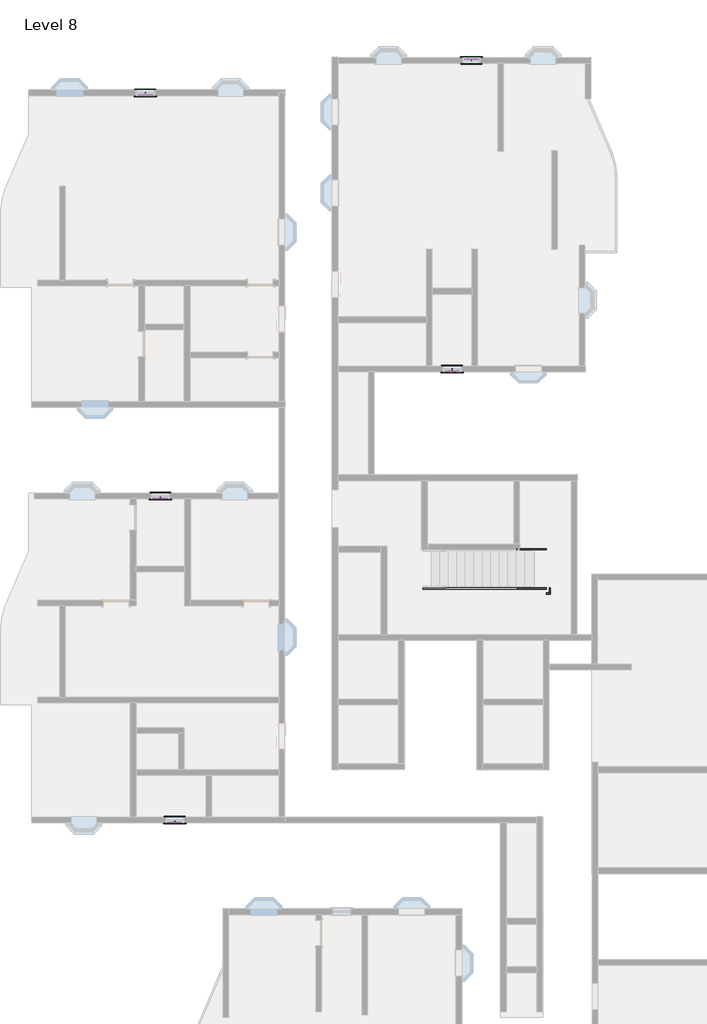
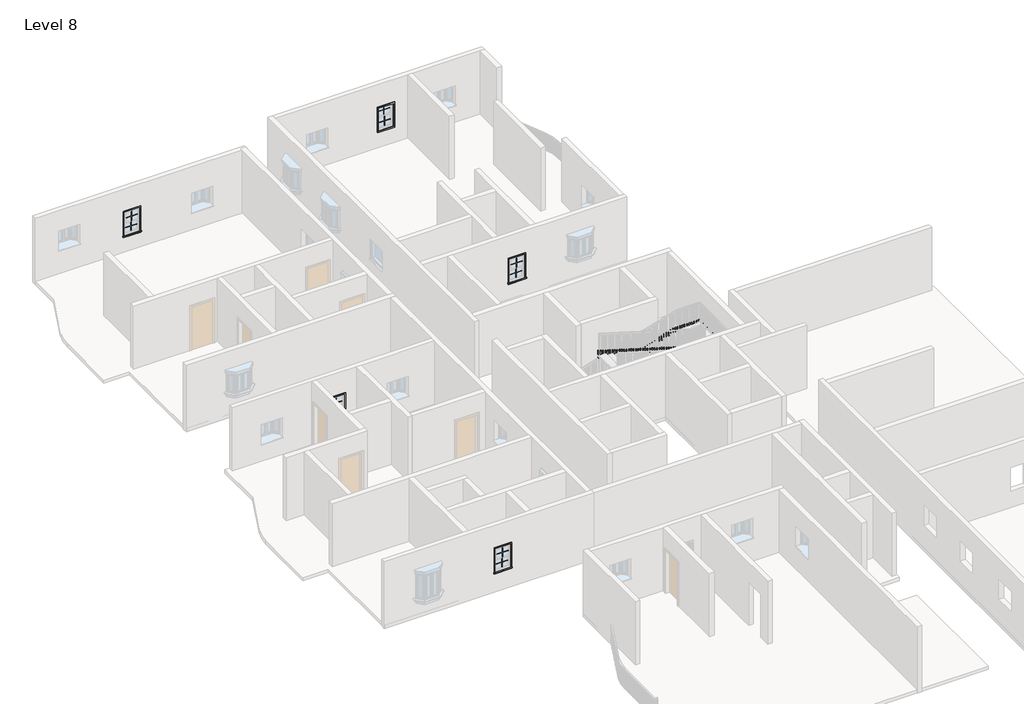
# One storey, part 14 of 14: 20 proxies, 6 members.
"""IFC4 building model written with IfcOpenShell, lengths in millimetres."""

from ifc_helpers import new_model, si_unit, frame, origin, place, context, project, spatial, polyline, outline, extrude, transform, mapped, element, save
from components import muntin_pattern_2x2_muntin_pattern_2x2_c35c595f, trim_window_exterior_flat_with_sill_e38017c9, trim_window_interior_flat_picture_frame_d728ed12

model = new_model("IFC4")

# Units and contexts
model_context = context("Model", 3, world=origin())
ifc_project = project(units=[si_unit("LENGTHUNIT", "METRE", prefix="MILLI")], contexts=[model_context])

# Site, building, storey
site = spatial("IfcSite", under=ifc_project)
building = spatial("IfcBuilding", under=site)
storey = spatial("IfcBuildingStorey", under=building, Name="Level 8", Elevation=21336.0)

# Proxies
placement = place(None, origin())
muntin_pattern_2x2_muntin_pattern_2x2_shape = muntin_pattern_2x2_muntin_pattern_2x2_c35c595f(model_context)
element("IfcBuildingElementProxy", 1, Name="Muntin Pattern_2x2 : Muntin Pattern_2x2", ObjectType="Muntin Pattern_2x2 : Muntin Pattern_2x2", at=placement, inside=storey, context=model_context, shape_type="MappedRepresentation", body=[
    mapped(muntin_pattern_2x2_muntin_pattern_2x2_shape, transform((-14639.3891351, 14368.0833494, 22806.025), x_axis=(-1.0, 0.0, 0.0), y_axis=(0.0, -1.0, 0.0), z_axis=(0.0, 0.0, 1.0))),
])
element("IfcBuildingElementProxy", 2, Name="Muntin Pattern_2x2 : Muntin Pattern_2x2", ObjectType="Muntin Pattern_2x2 : Muntin Pattern_2x2", at=placement, inside=storey, context=model_context, shape_type="MappedRepresentation", body=[
    mapped(muntin_pattern_2x2_muntin_pattern_2x2_shape, transform((-14639.3891351, 14412.5333494, 22326.6), x_axis=(-1.0, 0.0, 0.0), y_axis=(0.0, -1.0, 0.0), z_axis=(0.0, 0.0, 1.0))),
])
element("IfcBuildingElementProxy", 3, Name="Muntin Pattern_2x2 : Muntin Pattern_2x2", ObjectType="Muntin Pattern_2x2 : Muntin Pattern_2x2", at=placement, inside=storey, context=model_context, shape_type="MappedRepresentation", body=[
    mapped(muntin_pattern_2x2_muntin_pattern_2x2_shape, transform((-14125.0391351, 2785.6833494, 22806.025), x_axis=(-1.0, 0.0, 0.0), y_axis=(0.0, -1.0, 0.0), z_axis=(0.0, 0.0, 1.0))),
])
element("IfcBuildingElementProxy", 4, Name="Muntin Pattern_2x2 : Muntin Pattern_2x2", ObjectType="Muntin Pattern_2x2 : Muntin Pattern_2x2", at=placement, inside=storey, context=model_context, shape_type="MappedRepresentation", body=[
    mapped(muntin_pattern_2x2_muntin_pattern_2x2_shape, transform((-14125.0391351, 2830.1333494, 22326.6), x_axis=(-1.0, 0.0, 0.0), y_axis=(0.0, -1.0, 0.0), z_axis=(0.0, 0.0, 1.0))),
])
element("IfcBuildingElementProxy", 5, Name="Muntin Pattern_2x2 : Muntin Pattern_2x2", ObjectType="Muntin Pattern_2x2 : Muntin Pattern_2x2", at=placement, inside=storey, context=model_context, shape_type="MappedRepresentation", body=[
    mapped(muntin_pattern_2x2_muntin_pattern_2x2_shape, transform((-4206.3391351, 18910.0465905, 22806.025), x_axis=(-1.0, 0.0, 0.0), y_axis=(0.0, -1.0, 0.0), z_axis=(0.0, 0.0, 1.0))),
])
element("IfcBuildingElementProxy", 6, Name="Muntin Pattern_2x2 : Muntin Pattern_2x2", ObjectType="Muntin Pattern_2x2 : Muntin Pattern_2x2", at=placement, inside=storey, context=model_context, shape_type="MappedRepresentation", body=[
    mapped(muntin_pattern_2x2_muntin_pattern_2x2_shape, transform((-4206.3391351, 18954.4965905, 22326.6), x_axis=(-1.0, 0.0, 0.0), y_axis=(0.0, -1.0, 0.0), z_axis=(0.0, 0.0, 1.0))),
])
element("IfcBuildingElementProxy", 7, Name="Muntin Pattern_2x2 : Muntin Pattern_2x2", ObjectType="Muntin Pattern_2x2 : Muntin Pattern_2x2", at=placement, inside=storey, context=model_context, shape_type="MappedRepresentation", body=[
    mapped(muntin_pattern_2x2_muntin_pattern_2x2_shape, transform((-3514.1891351, 30066.9965905, 22806.025), x_axis=(1.0, 0.0, 0.0), y_axis=(0.0, 1.0, 0.0), z_axis=(0.0, 0.0, 1.0))),
])
element("IfcBuildingElementProxy", 8, Name="Muntin Pattern_2x2 : Muntin Pattern_2x2", ObjectType="Muntin Pattern_2x2 : Muntin Pattern_2x2", at=placement, inside=storey, context=model_context, shape_type="MappedRepresentation", body=[
    mapped(muntin_pattern_2x2_muntin_pattern_2x2_shape, transform((-3514.1891351, 30022.5465905, 22326.6), x_axis=(1.0, 0.0, 0.0), y_axis=(0.0, 1.0, 0.0), z_axis=(0.0, 0.0, 1.0))),
])
element("IfcBuildingElementProxy", 9, Name="Muntin Pattern_2x2 : Muntin Pattern_2x2", ObjectType="Muntin Pattern_2x2 : Muntin Pattern_2x2", at=placement, inside=storey, context=model_context, shape_type="MappedRepresentation", body=[
    mapped(muntin_pattern_2x2_muntin_pattern_2x2_shape, transform((-15175.9641351, 28782.5833494, 22806.025), x_axis=(-1.0, 0.0, 0.0), y_axis=(0.0, -1.0, 0.0), z_axis=(0.0, 0.0, 1.0))),
])
element("IfcBuildingElementProxy", 10, Name="Muntin Pattern_2x2 : Muntin Pattern_2x2", ObjectType="Muntin Pattern_2x2 : Muntin Pattern_2x2", at=placement, inside=storey, context=model_context, shape_type="MappedRepresentation", body=[
    mapped(muntin_pattern_2x2_muntin_pattern_2x2_shape, transform((-15175.9641351, 28827.0333494, 22326.6), x_axis=(-1.0, 0.0, 0.0), y_axis=(0.0, -1.0, 0.0), z_axis=(0.0, 0.0, 1.0))),
])
trim_window_exterior_flat_with_sill_shape = trim_window_exterior_flat_with_sill_e38017c9(model_context)
element("IfcBuildingElementProxy", 11, Name="Trim-Window-Exterior-Flat : with Sill", ObjectType="Trim-Window-Exterior-Flat : with Sill", at=placement, inside=storey, context=model_context, shape_type="MappedRepresentation", body=[
    mapped(trim_window_exterior_flat_with_sill_shape, transform((-14639.3891351, 14333.1583494, 23317.2), x_axis=(1.0, 0.0, 0.0), y_axis=(0.0, 0.0, 1.0), z_axis=(0.0, -1.0, 0.0))),
])
element("IfcBuildingElementProxy", 12, Name="Trim-Window-Exterior-Flat : with Sill", ObjectType="Trim-Window-Exterior-Flat : with Sill", at=placement, inside=storey, context=model_context, shape_type="MappedRepresentation", body=[
    mapped(trim_window_exterior_flat_with_sill_shape, transform((-14125.0391351, 2750.7583494, 23317.2), x_axis=(1.0, 0.0, 0.0), y_axis=(0.0, 0.0, 1.0), z_axis=(0.0, -1.0, 0.0))),
])
element("IfcBuildingElementProxy", 13, Name="Trim-Window-Exterior-Flat : with Sill", ObjectType="Trim-Window-Exterior-Flat : with Sill", at=placement, inside=storey, context=model_context, shape_type="MappedRepresentation", body=[
    mapped(trim_window_exterior_flat_with_sill_shape, transform((-4206.3391351, 18875.1215905, 23317.2), x_axis=(1.0, 0.0, 0.0), y_axis=(0.0, 0.0, 1.0), z_axis=(0.0, -1.0, 0.0))),
])
element("IfcBuildingElementProxy", 14, Name="Trim-Window-Exterior-Flat : with Sill", ObjectType="Trim-Window-Exterior-Flat : with Sill", at=placement, inside=storey, context=model_context, shape_type="MappedRepresentation", body=[
    mapped(trim_window_exterior_flat_with_sill_shape, transform((-3514.1891351, 30101.9215905, 23317.2), x_axis=(-1.0, 0.0, 0.0), y_axis=(0.0, 0.0, 1.0), z_axis=(0.0, 1.0, 0.0))),
])
element("IfcBuildingElementProxy", 15, Name="Trim-Window-Exterior-Flat : with Sill", ObjectType="Trim-Window-Exterior-Flat : with Sill", at=placement, inside=storey, context=model_context, shape_type="MappedRepresentation", body=[
    mapped(trim_window_exterior_flat_with_sill_shape, transform((-15175.9641351, 28747.6583494, 23317.2), x_axis=(1.0, 0.0, 0.0), y_axis=(0.0, 0.0, 1.0), z_axis=(0.0, -1.0, 0.0))),
])
trim_window_interior_flat_picture_frame_shape = trim_window_interior_flat_picture_frame_d728ed12(model_context)
element("IfcBuildingElementProxy", 16, Name="Trim-Window-Interior-Flat : Picture Frame", ObjectType="Trim-Window-Interior-Flat : Picture Frame", at=placement, inside=storey, context=model_context, shape_type="MappedRepresentation", body=[
    mapped(trim_window_interior_flat_picture_frame_shape, transform((-14639.3891351, 14536.3583494, 23317.2), x_axis=(-1.0, 0.0, 0.0), y_axis=(0.0, 0.0, 1.0), z_axis=(0.0, 1.0, 0.0))),
])
element("IfcBuildingElementProxy", 17, Name="Trim-Window-Interior-Flat : Picture Frame", ObjectType="Trim-Window-Interior-Flat : Picture Frame", at=placement, inside=storey, context=model_context, shape_type="MappedRepresentation", body=[
    mapped(trim_window_interior_flat_picture_frame_shape, transform((-14125.0391351, 2953.9583494, 23317.2), x_axis=(-1.0, 0.0, 0.0), y_axis=(0.0, 0.0, 1.0), z_axis=(0.0, 1.0, 0.0))),
])
element("IfcBuildingElementProxy", 18, Name="Trim-Window-Interior-Flat : Picture Frame", ObjectType="Trim-Window-Interior-Flat : Picture Frame", at=placement, inside=storey, context=model_context, shape_type="MappedRepresentation", body=[
    mapped(trim_window_interior_flat_picture_frame_shape, transform((-4206.3391351, 19078.3215905, 23317.2), x_axis=(-1.0, 0.0, 0.0), y_axis=(0.0, 0.0, 1.0), z_axis=(0.0, 1.0, 0.0))),
])
element("IfcBuildingElementProxy", 19, Name="Trim-Window-Interior-Flat : Picture Frame", ObjectType="Trim-Window-Interior-Flat : Picture Frame", at=placement, inside=storey, context=model_context, shape_type="MappedRepresentation", body=[
    mapped(trim_window_interior_flat_picture_frame_shape, transform((-3514.1891351, 29898.7215905, 23317.2), x_axis=(1.0, 0.0, 0.0), y_axis=(0.0, 0.0, 1.0), z_axis=(0.0, -1.0, 0.0))),
])
element("IfcBuildingElementProxy", 20, Name="Trim-Window-Interior-Flat : Picture Frame", ObjectType="Trim-Window-Interior-Flat : Picture Frame", at=placement, inside=storey, context=model_context, shape_type="MappedRepresentation", body=[
    mapped(trim_window_interior_flat_picture_frame_shape, transform((-15175.9641351, 28950.8583494, 23317.2), x_axis=(-1.0, 0.0, 0.0), y_axis=(0.0, 0.0, 1.0), z_axis=(0.0, 1.0, 0.0))),
])

# Members
element("IfcMember", 21, ObjectType="Stringer - 2\" Width", at=placement, inside=storey, context=model_context, shape_type="SweptSolid", body=[
    extrude(outline(polyline([(21527.5995961, -5254.0891351), (21336.0, -5254.0891351), (21336.0, -4832.019314), (22783.8, -6.019314), (22783.8, -1066.7544553), (21527.5995961, -5254.0891351)])), frame((0.0, 12506.0715905, 0.0), z_axis=(0.0, 1.0, 0.0), x_axis=(0.0, 0.0, 1.0)), (0.0, 0.0, 1.0), 50.8),
])
element("IfcMember", 22, ObjectType="Stringer - 2\" Width", at=placement, inside=storey, context=model_context, shape_type="SweptSolid", body=[
    extrude(outline(polyline([(54.5108649, 12556.8715905), (105.3108649, 12556.8715905), (105.3108649, 9478.4949943), (54.5108649, 9478.4949943), (54.5108649, 12556.8715905)])), frame((0.0, 0.0, 22479.0), z_axis=(0.0, 0.0, 1.0), x_axis=(1.0, 0.0, 0.0)), (0.0, 0.0, 1.0), 304.8),
])
element("IfcMember", 23, ObjectType="Stringer - 2\" Width", at=placement, inside=storey, context=model_context, shape_type="SweptSolid", body=[
    extrude(outline(polyline([(22479.0, 105.3108649), (22571.5395961, 105.3108649), (24179.3595961, -5254.0891351), (23861.1390537, -5254.0891351), (22479.0, -646.9589562), (22479.0, 105.3108649)])), frame((0.0, 9427.6949943, 0.0), z_axis=(0.0, 1.0, 0.0), x_axis=(0.0, 0.0, 1.0)), (0.0, 0.0, 1.0), 50.8),
])
element("IfcMember", 24, ObjectType="Stringer - 2\" Width", at=placement, inside=storey, context=model_context, shape_type="SweptSolid", body=[
    extrude(outline(polyline([(21527.5995961, -5254.0891351), (21336.0, -5254.0891351), (21336.0, -4832.019314), (22565.7390537, -732.8891351), (22783.8, -732.8891351), (22783.8, -1066.7544553), (21527.5995961, -5254.0891351)])), frame((0.0, 11103.4082924, 0.0), z_axis=(0.0, 1.0, 0.0), x_axis=(0.0, 0.0, 1.0)), (0.0, 0.0, 1.0), 50.8),
])
element("IfcMember", 25, ObjectType="Stringer - 2\" Width", at=placement, inside=storey, context=model_context, shape_type="SweptSolid", body=[
    extrude(outline(polyline([(-732.8891351, 11154.2082924), (-682.0891351, 11154.2082924), (-682.0891351, 10976.4082924), (-732.8891351, 10976.4082924), (-732.8891351, 11154.2082924)])), frame((0.0, 0.0, 22479.0), z_axis=(0.0, 0.0, 1.0), x_axis=(1.0, 0.0, 0.0)), (0.0, 0.0, 1.0), 304.8),
])
element("IfcMember", 26, ObjectType="Stringer - 2\" Width", at=placement, inside=storey, context=model_context, shape_type="SweptSolid", body=[
    extrude(outline(polyline([(22489.5390537, -682.0891351), (22807.7595961, -682.0891351), (24179.3595961, -5254.0891351), (23861.1390537, -5254.0891351), (22489.5390537, -682.0891351)])), frame((0.0, 10925.6082924, 0.0), z_axis=(0.0, 1.0, 0.0), x_axis=(0.0, 0.0, 1.0)), (0.0, 0.0, 1.0), 50.8),
])

save(model, "model.ifc")

# Revit data of these elements
# Type "Muntin Pattern_2x2 : Muntin Pattern_2x2"
#   Width [instance default] = 4' - 0"
#   Thickness = 0' - 0 1/2"
#   Height [instance default] = 4' - 0"
#   Distance = 0' - 0 3/4"
#   Interior Material [instance default] = none
#   Exterior Material [instance default] = none
#   Default Elevation = 0
# Type "Trim-Window-Exterior-Flat : with Sill"
#   Trim Width = 0' - 2 1/4"
#   Trim Thickness_Picture Frame = 0' - 1 1/4"
#   Trim Thickness_with Sill = 0' - 0 3/4"
#   Sill Thickness = 0' - 1 1/4"
#   Opening Width [instance default] = 2' - 0"
#   Opening Height [instance default] = 3' - 0"
#   Default Elevation = 4' - 0"
#   Sill = yes
#   Picture Frame = no
#   Trim Material [instance default] = none
# Type "Trim-Window-Interior-Flat : Picture Frame"
#   Trim Thickness_Picture Frame = 0' - 1 1/4"
#   Trim Width = 0' - 2 1/4"
#   Trim Thickness_with Sill = 0' - 0 3/4"
#   Sill Thickness = 0' - 1 1/4"
#   Opening Width [instance default] = 2' - 0"
#   Opening Height [instance default] = 3' - 0"
#   Default Elevation = 4' - 0"
#   Sill = no
#   Picture Frame = yes
#   Trim Material [instance default] = none
# Elements 1, 2, 3, 4, 5, 6, 7, 8, 9, 10 (IfcBuildingElementProxy, "Muntin Pattern_2x2 : Muntin Pattern_2x2")
#   Width = 1' - 8"
#   Height = 1' - 5 1/8"
#   Interior Material = Wood - Stained
#   Exterior Material = Clad - White
#   Phase Created = New Construction
#   Materials on its faces: "Clad - White", "Wood - Stained"
# Elements 11, 12, 13, 14, 15 (IfcBuildingElementProxy, "Trim-Window-Exterior-Flat : with Sill")
#   Opening Width = 2' - 2"
#   Opening Height = 3' - 6"
#   Trim Material = Clad - White
#   Phase Created = New Construction
#   Materials on its faces: "Clad - White"
# Elements 16, 17, 18, 19, 20 (IfcBuildingElementProxy, "Trim-Window-Interior-Flat : Picture Frame")
#   Opening Width = 2' - 2"
#   Opening Height = 3' - 6"
#   Trim Material = Wood - Stained
#   Phase Created = New Construction
#   Materials on its faces: "Wood - Stained"
# Elements 21, 22, 23, 24, 25, 26 (IfcMember, "Stringer - 2\" Width")
#   Phase Created = New Construction
# Materials
#   "Clad - White": class "Wood", colour RGB 242 242 238, transparency 0, Cost = 0
#   "Wood - Stained": class "Wood", colour RGB 224 178 126, transparency 0, Cost = 0
